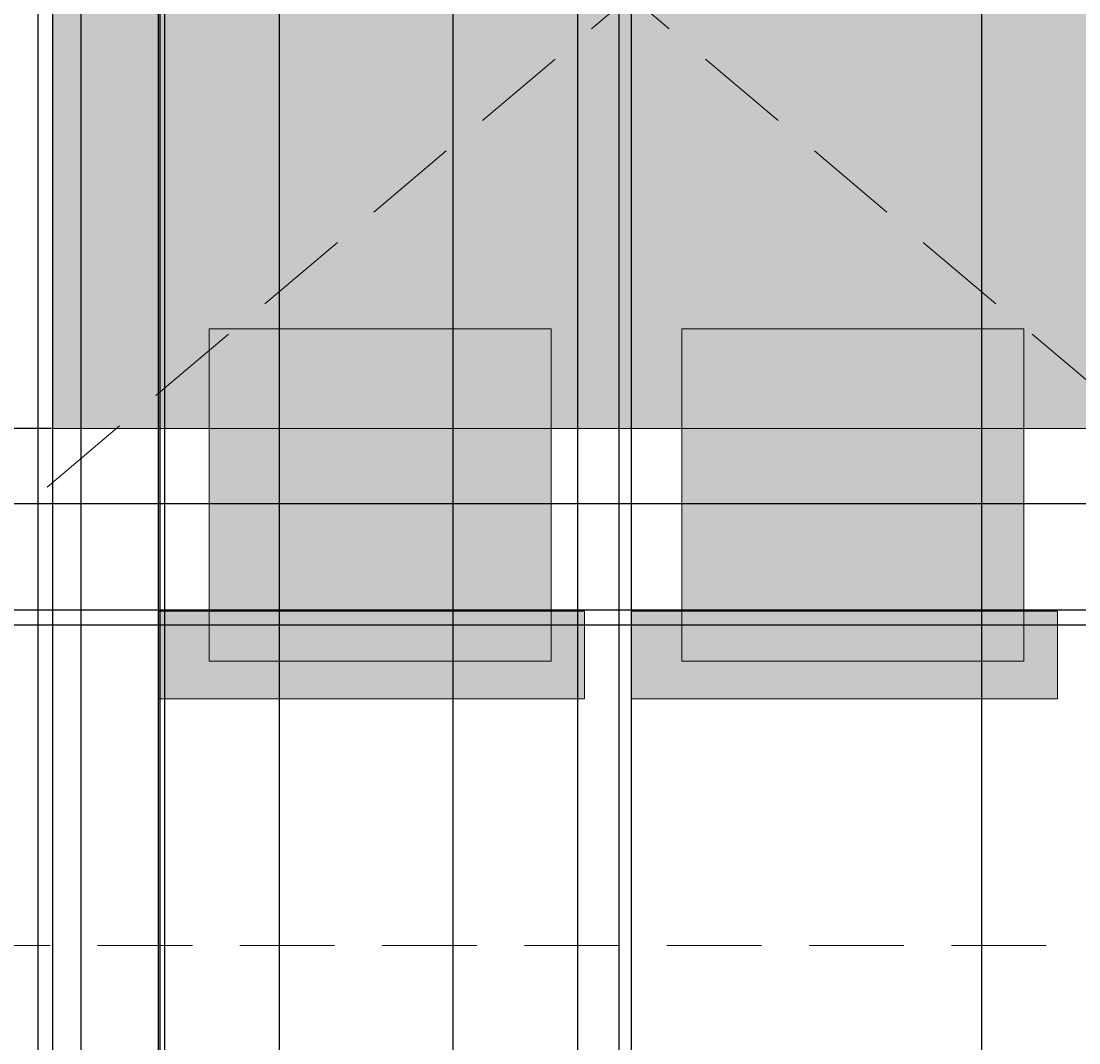
# Model space of a CAD drawing. Units: inches. Extents: x 818 to 1898, y 976 to 2364.
# Tile 69 of 96: x 1302 to 1372, y 1913 to 1980. Entities that reach past the tile are written whole.
import ezdxf

# ---------------------------------------------------------------- set-up
doc = ezdxf.new("R2010")
doc.units = ezdxf.units.IN
doc.header["$LTSCALE"] = 5
doc.header["$MEASUREMENT"] = 0
doc.linetypes.add('HIDDEN', pattern=[0.375, 0.25, -0.125])
for name, color, linetype, lineweight in [('A-ANNO-DIMS', 2, 'Continuous', 18), ('A-FLOR-OVHD', 8, 'HIDDEN', 13), ('A-FURN', 8, 'Continuous', 18), ('A-FURN-PATT', 8, 'Continuous', 9)]:
    doc.layers.add(name, color=color, linetype=linetype, lineweight=lineweight)
doc.styles.get("Standard").update_dxf_attribs({"font": 'arial.ttf'})
doc.dimstyles.get("Standard").update_dxf_attribs({"dimtxt": 0.18, "dimasz": 0.18, "dimexe": 0.18, "dimexo": 0.0625, "dimgap": 0.09, "dimtad": 0, "dimtih": 1, "dimtoh": 1, "dimdec": 4, "dimzin": 0, "dimdsep": 46, "dimtxsty": 'Standard', "dimcen": 0.09, "dimadec": 0, "dimazin": 0, "dimtfac": 1, "dimtdec": 4, "dimtofl": 0, "dimtmove": 0, "dimatfit": 3, "dimfxl": 1, "dimtolj": 1, "dimtzin": 0, "dimarcsym": 0})

# ---------------------------------------------------------------- blocks, each defined once
blk = doc.blocks.new('*D61')
at = {"layer": 'A-ANNO-DIMS', "color": 0, "lineweight": -2, "ltscale": 5, "transparency": 16777216}
for p, q in [((1071.725, 1203.027), (1071.725, 2363.873)), ((1071.905, 2363.693), (1250.936, 2363.693)), ((1430.545, 2363.693), (1251.514, 2363.693)), ((1430.725, 1203.027), (1430.725, 2363.873))]:
    blk.add_line(p, q, dxfattribs=at)
at = {"layer": 'A-ANNO-DIMS', "color": 0, "ltscale": 5, "transparency": 16777216}
for points in [[(1071.905, 2363.723), (1071.905, 2363.663), (1071.725, 2363.693)], [(1430.545, 2363.723), (1430.545, 2363.663), (1430.725, 2363.693)]]:
    blk.add_solid(points, dxfattribs=at)
at = {"layer": 'Defpoints', "color": 0, "ltscale": 5, "transparency": 16777216}
for p in [(1430.725, 2363.693), (1071.725, 1202.964), (1430.725, 1202.964)]:
    blk.add_point(p, dxfattribs=at)
at = {"layer": 'A-ANNO-DIMS', "color": 0, "ltscale": 5, "transparency": 16777216, "insert": (1251.225, 2363.693), "char_height": 0.18, "attachment_point": 5}
blk.add_mtext('\\A1;359', dxfattribs=at)
blk = doc.blocks.new('*D64')
at = {"layer": 'A-ANNO-DIMS', "color": 0, "lineweight": -2, "ltscale": 5, "transparency": 16777216}
for p, q in [((1197.725, 1501.141), (1197.725, 2363.873)), ((1197.905, 2363.693), (1313.935, 2363.693)), ((1430.545, 2363.693), (1314.516, 2363.693)), ((1430.725, 1501.141), (1430.725, 2363.873))]:
    blk.add_line(p, q, dxfattribs=at)
at = {"layer": 'A-ANNO-DIMS', "color": 0, "ltscale": 5, "transparency": 16777216}
for points in [[(1197.905, 2363.723), (1197.905, 2363.663), (1197.725, 2363.693)], [(1430.545, 2363.723), (1430.545, 2363.663), (1430.725, 2363.693)]]:
    blk.add_solid(points, dxfattribs=at)
at = {"layer": 'Defpoints', "color": 0, "ltscale": 5, "transparency": 16777216}
for p in [(1430.725, 2363.693), (1197.725, 1501.078), (1430.725, 1501.078)]:
    blk.add_point(p, dxfattribs=at)
at = {"layer": 'A-ANNO-DIMS', "color": 0, "ltscale": 5, "transparency": 16777216, "insert": (1314.225, 2363.693), "char_height": 0.18, "attachment_point": 5}
blk.add_mtext('\\A1;233', dxfattribs=at)
blk = doc.blocks.new('*D74')
at = {"layer": 'A-ANNO-DIMS', "color": 0, "lineweight": -2, "ltscale": 5, "transparency": 16777216}
for p, q in [((1590.663, 1940.078), (818.026, 1940.078)), ((818.206, 1939.898), (818.206, 1925.76)), ((818.206, 1911.258), (818.206, 1925.396)), ((1590.663, 1911.078), (818.026, 1911.078))]:
    blk.add_line(p, q, dxfattribs=at)
at = {"layer": 'A-ANNO-DIMS', "color": 0, "ltscale": 5, "transparency": 16777216}
for points in [[(818.176, 1939.898), (818.236, 1939.898), (818.206, 1940.078)], [(818.176, 1911.258), (818.236, 1911.258), (818.206, 1911.078)]]:
    blk.add_solid(points, dxfattribs=at)
at = {"layer": 'Defpoints', "color": 0, "ltscale": 5, "transparency": 16777216}
for p in [(818.206, 1940.078), (1590.725, 1940.078), (1590.725, 1911.078)]:
    blk.add_point(p, dxfattribs=at)
at = {"layer": 'A-ANNO-DIMS', "color": 0, "ltscale": 5, "transparency": 16777216, "insert": (818.206, 1925.578), "char_height": 0.18, "attachment_point": 5}
blk.add_mtext('\\A1;29', dxfattribs=at)
blk = doc.blocks.new('*D85')
at = {"layer": 'A-ANNO-DIMS', "color": 0, "lineweight": -2, "ltscale": 5, "transparency": 16777216}
for p, q in [((1258.788, 2053.078), (1897.916, 2053.078)), ((1897.736, 2052.898), (1897.736, 1876.76)), ((1897.736, 1700.258), (1897.736, 1876.396)), ((1258.788, 1700.078), (1897.916, 1700.078))]:
    blk.add_line(p, q, dxfattribs=at)
at = {"layer": 'A-ANNO-DIMS', "color": 0, "ltscale": 5, "transparency": 16777216}
for points in [[(1897.706, 2052.898), (1897.766, 2052.898), (1897.736, 2053.078)], [(1897.706, 1700.258), (1897.766, 1700.258), (1897.736, 1700.078)]]:
    blk.add_solid(points, dxfattribs=at)
at = {"layer": 'Defpoints', "color": 0, "ltscale": 5, "transparency": 16777216}
for p in [(1258.725, 2053.078), (1897.736, 2053.078), (1258.725, 1700.078)]:
    blk.add_point(p, dxfattribs=at)
at = {"layer": 'A-ANNO-DIMS', "color": 0, "ltscale": 5, "transparency": 16777216, "insert": (1897.736, 1876.578), "char_height": 0.18, "attachment_point": 5}
blk.add_mtext('\\A1;353', dxfattribs=at)
blk = doc.blocks.new('*D97')
at = {"layer": 'A-ANNO-DIMS', "color": 0, "lineweight": -2, "ltscale": 5, "transparency": 16777216}
for p, q in [((1284.17, 1071.118), (1284.17, 2363.873)), ((1284.35, 2363.693), (1310.962, 2363.693)), ((1338.361, 2363.693), (1311.749, 2363.693)), ((1338.541, 1071.118), (1338.541, 2363.873))]:
    blk.add_line(p, q, dxfattribs=at)
at = {"layer": 'A-ANNO-DIMS', "color": 0, "ltscale": 5, "transparency": 16777216}
for points in [[(1284.35, 2363.723), (1284.35, 2363.663), (1284.17, 2363.693)], [(1338.361, 2363.723), (1338.361, 2363.663), (1338.541, 2363.693)]]:
    blk.add_solid(points, dxfattribs=at)
at = {"layer": 'Defpoints', "color": 0, "ltscale": 5, "transparency": 16777216}
for p in [(1338.541, 2363.693), (1284.17, 1071.055), (1338.541, 1071.055)]:
    blk.add_point(p, dxfattribs=at)
at = {"layer": 'A-ANNO-DIMS', "color": 0, "ltscale": 5, "transparency": 16777216, "insert": (1311.355, 2363.693), "char_height": 0.18, "attachment_point": 5}
blk.add_mtext('\\A1;54.37', dxfattribs=at)
blk = doc.blocks.new('*D98')
at = {"layer": 'A-ANNO-DIMS', "color": 0, "lineweight": -2, "ltscale": 5, "transparency": 16777216}
for p, q in [((1338.541, 1071.118), (1338.541, 2363.873)), ((1338.721, 2363.693), (1364.815, 2363.693)), ((1391.696, 2363.693), (1365.602, 2363.693)), ((1391.876, 1071.118), (1391.876, 2363.873))]:
    blk.add_line(p, q, dxfattribs=at)
at = {"layer": 'A-ANNO-DIMS', "color": 0, "ltscale": 5, "transparency": 16777216}
for points in [[(1338.721, 2363.723), (1338.721, 2363.663), (1338.541, 2363.693)], [(1391.696, 2363.723), (1391.696, 2363.663), (1391.876, 2363.693)]]:
    blk.add_solid(points, dxfattribs=at)
at = {"layer": 'Defpoints', "color": 0, "ltscale": 5, "transparency": 16777216}
for p in [(1391.876, 2363.693), (1338.541, 1071.055), (1391.876, 1071.055)]:
    blk.add_point(p, dxfattribs=at)
at = {"layer": 'A-ANNO-DIMS', "color": 0, "ltscale": 5, "transparency": 16777216, "insert": (1365.208, 2363.693), "char_height": 0.18, "attachment_point": 5}
blk.add_mtext('\\A1;53.33', dxfattribs=at)
blk = doc.blocks.new('*D165')
at = {"layer": 'A-ANNO-DIMS', "color": 0, "lineweight": -2, "ltscale": 5, "transparency": 16777216}
for p, q in [((1283.818, 1510.141), (1283.818, 2363.873)), ((1283.998, 2363.693), (1324.088, 2363.693)), ((1364.966, 2363.693), (1324.876, 2363.693)), ((1365.146, 1510.141), (1365.146, 2363.873))]:
    blk.add_line(p, q, dxfattribs=at)
at = {"layer": 'A-ANNO-DIMS', "color": 0, "ltscale": 5, "transparency": 16777216}
for points in [[(1283.998, 2363.723), (1283.998, 2363.663), (1283.818, 2363.693)], [(1364.966, 2363.723), (1364.966, 2363.663), (1365.146, 2363.693)]]:
    blk.add_solid(points, dxfattribs=at)
at = {"layer": 'Defpoints', "color": 0, "ltscale": 5, "transparency": 16777216}
for p in [(1365.146, 2363.693), (1283.818, 1510.078), (1365.146, 1510.078)]:
    blk.add_point(p, dxfattribs=at)
at = {"layer": 'A-ANNO-DIMS', "color": 0, "ltscale": 5, "transparency": 16777216, "insert": (1324.482, 2363.693), "char_height": 0.18, "attachment_point": 5}
blk.add_mtext('\\A1;81.33', dxfattribs=at)
blk = doc.blocks.new('*D211')
at = {"layer": 'A-ANNO-DIMS', "color": 0, "lineweight": -2, "ltscale": 5, "transparency": 16777216}
for p, q in [((1599.66265, 1948.078237), (818.025912, 1948.078237)), ((818.205912, 1947.898237), (818.205912, 1944.758237)), ((818.205912, 1941.258237), (818.205912, 1944.398237)), ((1599.66265, 1941.078237), (818.025912, 1941.078237))]:
    blk.add_line(p, q, dxfattribs=at)
at = {"layer": 'A-ANNO-DIMS', "color": 0, "ltscale": 5, "transparency": 16777216}
for points in [[(818.175912, 1947.898237), (818.235912, 1947.898237), (818.205912, 1948.078237)], [(818.175912, 1941.258237), (818.235912, 1941.258237), (818.205912, 1941.078237)]]:
    blk.add_solid(points, dxfattribs=at)
at = {"layer": 'Defpoints', "color": 0, "ltscale": 5, "transparency": 16777216}
for p in [(818.205912, 1948.078237), (1599.72515, 1948.078237), (1599.72515, 1941.078237)]:
    blk.add_point(p, dxfattribs=at)
at = {"layer": 'A-ANNO-DIMS', "color": 0, "ltscale": 5, "transparency": 16777216, "insert": (818.205912, 1944.578237), "char_height": 0.18, "attachment_point": 5}
blk.add_mtext('\\A1;7', dxfattribs=at)
blk = doc.blocks.new('*D231')
at = {"layer": 'A-ANNO-DIMS', "color": 0, "lineweight": -2, "ltscale": 5, "transparency": 16777216}
for p, q in [((1303.931, 1952.978), (1303.931, 975.663)), ((1402.518, 1952.978), (1402.518, 975.663)), ((1304.111, 975.843), (1352.831, 975.843)), ((1402.338, 975.843), (1353.619, 975.843))]:
    blk.add_line(p, q, dxfattribs=at)
at = {"layer": 'A-ANNO-DIMS', "color": 0, "ltscale": 5, "transparency": 16777216}
for points in [[(1304.111, 975.873), (1304.111, 975.813), (1303.931, 975.843)], [(1402.338, 975.873), (1402.338, 975.813), (1402.518, 975.843)]]:
    blk.add_solid(points, dxfattribs=at)
at = {"layer": 'Defpoints', "color": 0, "ltscale": 5, "transparency": 16777216}
for p in [(1303.931, 1953.041), (1402.518, 1953.041), (1402.518, 975.843)]:
    blk.add_point(p, dxfattribs=at)
at = {"layer": 'A-ANNO-DIMS', "color": 0, "ltscale": 5, "transparency": 16777216, "insert": (1353.225, 975.843), "char_height": 0.18, "attachment_point": 5}
blk.add_mtext('\\A1;98.59', dxfattribs=at)
blk = doc.blocks.new('*D232')
at = {"layer": 'A-ANNO-DIMS', "color": 0, "lineweight": -2, "ltscale": 5, "transparency": 16777216}
for p, q in [((1303.869, 2008.392), (818.026, 2008.392)), ((818.206, 2008.212), (818.206, 1980.898)), ((818.206, 1953.221), (818.206, 1980.534)), ((1303.869, 1953.041), (818.026, 1953.041))]:
    blk.add_line(p, q, dxfattribs=at)
at = {"layer": 'A-ANNO-DIMS', "color": 0, "ltscale": 5, "transparency": 16777216}
for points in [[(818.176, 2008.212), (818.236, 2008.212), (818.206, 2008.392)], [(818.176, 1953.221), (818.236, 1953.221), (818.206, 1953.041)]]:
    blk.add_solid(points, dxfattribs=at)
at = {"layer": 'Defpoints', "color": 0, "ltscale": 5, "transparency": 16777216}
for p in [(818.206, 2008.392), (1303.931, 2008.392), (1303.931, 1953.041)]:
    blk.add_point(p, dxfattribs=at)
at = {"layer": 'A-ANNO-DIMS', "color": 0, "ltscale": 5, "transparency": 16777216, "insert": (818.206, 1980.716), "char_height": 0.18, "attachment_point": 5}
blk.add_mtext('\\A1;55.35', dxfattribs=at)
blk = doc.blocks.new('*D233')
at = {"layer": 'A-ANNO-DIMS', "color": 0, "lineweight": -2, "ltscale": 5, "transparency": 16777216}
for p, q in [((1267.725, 2044.016), (1267.725, 975.663)), ((1303.931, 2008.329), (1303.931, 975.663)), ((1267.905, 975.843), (1285.365, 975.843)), ((1303.751, 975.843), (1286.292, 975.843))]:
    blk.add_line(p, q, dxfattribs=at)
at = {"layer": 'A-ANNO-DIMS', "color": 0, "ltscale": 5, "transparency": 16777216}
for points in [[(1267.905, 975.873), (1267.905, 975.813), (1267.725, 975.843)], [(1303.751, 975.873), (1303.751, 975.813), (1303.931, 975.843)]]:
    blk.add_solid(points, dxfattribs=at)
at = {"layer": 'Defpoints', "color": 0, "ltscale": 5, "transparency": 16777216}
for p in [(1267.725, 2044.078), (1303.931, 2008.392), (1303.931, 975.843)]:
    blk.add_point(p, dxfattribs=at)
at = {"layer": 'A-ANNO-DIMS', "color": 0, "ltscale": 5, "transparency": 16777216, "insert": (1285.828, 975.843), "char_height": 0.18, "attachment_point": 5}
blk.add_mtext('\\A1;36.206', dxfattribs=at)
blk = doc.blocks.new('*D236')
at = {"layer": 'A-ANNO-DIMS', "color": 0, "lineweight": -2, "ltscale": 5, "transparency": 16777216}
for p, q in [((1310.908, 2026.145), (1310.908, 975.663)), ((1342.045, 2026.145), (1342.045, 975.663)), ((1311.088, 975.843), (1326.083, 975.843)), ((1341.865, 975.843), (1326.87, 975.843))]:
    blk.add_line(p, q, dxfattribs=at)
at = {"layer": 'A-ANNO-DIMS', "color": 0, "ltscale": 5, "transparency": 16777216}
for points in [[(1311.088, 975.873), (1311.088, 975.813), (1310.908, 975.843)], [(1341.865, 975.873), (1341.865, 975.813), (1342.045, 975.843)]]:
    blk.add_solid(points, dxfattribs=at)
at = {"layer": 'Defpoints', "color": 0, "ltscale": 5, "transparency": 16777216}
for p in [(1310.908, 2026.207), (1342.045, 2026.207), (1342.045, 975.843)]:
    blk.add_point(p, dxfattribs=at)
at = {"layer": 'A-ANNO-DIMS', "color": 0, "ltscale": 5, "transparency": 16777216, "insert": (1326.476, 975.843), "char_height": 0.18, "attachment_point": 5}
blk.add_mtext('\\A1;31.14', dxfattribs=at)
blk = doc.blocks.new('*D252')
at = {"layer": 'A-ANNO-DIMS', "color": 0, "lineweight": -2, "ltscale": 5, "transparency": 16777216}
for p, q in [((1330.305, 2053.016), (1330.305, 975.663)), ((1388.031, 2053.016), (1388.031, 975.663)), ((1330.485, 975.843), (1358.775, 975.843)), ((1387.851, 975.843), (1359.562, 975.843))]:
    blk.add_line(p, q, dxfattribs=at)
at = {"layer": 'A-ANNO-DIMS', "color": 0, "ltscale": 5, "transparency": 16777216}
for points in [[(1330.485, 975.873), (1330.485, 975.813), (1330.305, 975.843)], [(1387.851, 975.873), (1387.851, 975.813), (1388.031, 975.843)]]:
    blk.add_solid(points, dxfattribs=at)
at = {"layer": 'Defpoints', "color": 0, "ltscale": 5, "transparency": 16777216}
for p in [(1330.305, 2053.078), (1388.031, 2053.078), (1388.031, 975.843)]:
    blk.add_point(p, dxfattribs=at)
at = {"layer": 'A-ANNO-DIMS', "color": 0, "ltscale": 5, "transparency": 16777216, "insert": (1359.168, 975.843), "char_height": 0.18, "attachment_point": 5}
blk.add_mtext('\\A1;57.73', dxfattribs=at)
blk = doc.blocks.new('*D254')
at = {"layer": 'A-ANNO-DIMS', "color": 0, "lineweight": -2, "ltscale": 5, "transparency": 16777216}
for p, q in [((1267.725, 2044.016), (1267.725, 975.663)), ((1330.305, 2044.016), (1330.305, 975.663)), ((1267.905, 975.843), (1298.621, 975.843)), ((1330.125, 975.843), (1299.409, 975.843))]:
    blk.add_line(p, q, dxfattribs=at)
at = {"layer": 'A-ANNO-DIMS', "color": 0, "ltscale": 5, "transparency": 16777216}
for points in [[(1267.905, 975.873), (1267.905, 975.813), (1267.725, 975.843)], [(1330.125, 975.873), (1330.125, 975.813), (1330.305, 975.843)]]:
    blk.add_solid(points, dxfattribs=at)
at = {"layer": 'Defpoints', "color": 0, "ltscale": 5, "transparency": 16777216}
for p in [(1267.725, 2044.078), (1330.305, 2044.078), (1330.305, 975.843)]:
    blk.add_point(p, dxfattribs=at)
at = {"layer": 'A-ANNO-DIMS', "color": 0, "ltscale": 5, "transparency": 16777216, "insert": (1299.015, 975.843), "char_height": 0.18, "attachment_point": 5}
blk.add_mtext('\\A1;62.58', dxfattribs=at)
blk = doc.blocks.new('*D269')
at = {"layer": 'A-ANNO-DIMS', "color": 0, "lineweight": -2, "ltscale": 5, "transparency": 16777216}
for p, q in [((1246.938, 1534.141), (1246.938, 2363.873)), ((1247.118, 2363.693), (1293.706, 2363.693)), ((1341.079, 2363.693), (1294.491, 2363.693)), ((1341.259, 1534.141), (1341.259, 2363.873))]:
    blk.add_line(p, q, dxfattribs=at)
at = {"layer": 'A-ANNO-DIMS', "color": 0, "ltscale": 5, "transparency": 16777216}
for points in [[(1247.118, 2363.723), (1247.118, 2363.663), (1246.938, 2363.693)], [(1341.079, 2363.723), (1341.079, 2363.663), (1341.259, 2363.693)]]:
    blk.add_solid(points, dxfattribs=at)
at = {"layer": 'Defpoints', "color": 0, "ltscale": 5, "transparency": 16777216}
for p in [(1341.259, 2363.693), (1246.938, 1534.078), (1341.259, 1534.078)]:
    blk.add_point(p, dxfattribs=at)
at = {"layer": 'A-ANNO-DIMS', "color": 0, "ltscale": 5, "transparency": 16777216, "insert": (1294.099, 2363.693), "char_height": 0.18, "attachment_point": 5}
blk.add_mtext('\\A1;94.32', dxfattribs=at)
blk = doc.blocks.new('*D274')
at = {"layer": 'A-ANNO-DIMS', "color": 0, "lineweight": -2, "ltscale": 5, "transparency": 16777216}
for p, q in [((1311.025, 1897.929), (1311.025, 2363.873)), ((1311.205, 2363.693), (1344.007, 2363.693)), ((1377.599, 2363.693), (1344.797, 2363.693)), ((1377.779, 1897.929), (1377.779, 2363.873))]:
    blk.add_line(p, q, dxfattribs=at)
at = {"layer": 'A-ANNO-DIMS', "color": 0, "ltscale": 5, "transparency": 16777216}
for points in [[(1311.205, 2363.723), (1311.205, 2363.663), (1311.025, 2363.693)], [(1377.599, 2363.723), (1377.599, 2363.663), (1377.779, 2363.693)]]:
    blk.add_solid(points, dxfattribs=at)
at = {"layer": 'Defpoints', "color": 0, "ltscale": 5, "transparency": 16777216}
for p in [(1377.779, 2363.693), (1311.025, 1897.866), (1377.779, 1897.866)]:
    blk.add_point(p, dxfattribs=at)
at = {"layer": 'A-ANNO-DIMS', "color": 0, "ltscale": 5, "transparency": 16777216, "insert": (1344.402, 2363.693), "char_height": 0.18, "attachment_point": 5}
blk.add_mtext('\\A1;66.75', dxfattribs=at)
blk = doc.blocks.new('*D281')
at = {"layer": 'A-ANNO-DIMS', "color": 0, "lineweight": -2, "ltscale": 5, "transparency": 16777216}
for p, q in [((1250.303, 1913.703), (1250.303, 2363.873)), ((1250.483, 2363.693), (1420.121, 2363.693)), ((1590.545, 2363.693), (1420.907, 2363.693)), ((1590.725, 2011.141), (1590.725, 2363.873))]:
    blk.add_line(p, q, dxfattribs=at)
at = {"layer": 'A-ANNO-DIMS', "color": 0, "ltscale": 5, "transparency": 16777216}
for points in [[(1250.483, 2363.723), (1250.483, 2363.663), (1250.303, 2363.693)], [(1590.545, 2363.723), (1590.545, 2363.663), (1590.725, 2363.693)]]:
    blk.add_solid(points, dxfattribs=at)
at = {"layer": 'Defpoints', "color": 0, "ltscale": 5, "transparency": 16777216}
for p in [(1590.725, 2363.693), (1590.725, 2011.078), (1250.303, 1913.64)]:
    blk.add_point(p, dxfattribs=at)
at = {"layer": 'A-ANNO-DIMS', "color": 0, "ltscale": 5, "transparency": 16777216, "insert": (1420.514, 2363.693), "char_height": 0.18, "attachment_point": 5}
blk.add_mtext('\\A1;340.4', dxfattribs=at)
blk = doc.blocks.new('*D286')
at = {"layer": 'A-ANNO-DIMS', "color": 0, "lineweight": -2, "ltscale": 5, "transparency": 16777216}
for p, q in [((1305.828, 1851.971), (1305.828, 2363.873)), ((1306.008, 2363.693), (1308.184, 2363.693)), ((1311.147, 2363.693), (1308.971, 2363.693)), ((1311.327, 1853.812), (1311.327, 2363.873))]:
    blk.add_line(p, q, dxfattribs=at)
at = {"layer": 'A-ANNO-DIMS', "color": 0, "ltscale": 5, "transparency": 16777216}
for points in [[(1306.008, 2363.723), (1306.008, 2363.663), (1305.828, 2363.693)], [(1311.147, 2363.723), (1311.147, 2363.663), (1311.327, 2363.693)]]:
    blk.add_solid(points, dxfattribs=at)
at = {"layer": 'Defpoints', "color": 0, "ltscale": 5, "transparency": 16777216}
for p in [(1305.828, 2363.693), (1311.327, 1853.75), (1305.828, 1851.908)]:
    blk.add_point(p, dxfattribs=at)
at = {"layer": 'A-ANNO-DIMS', "color": 0, "ltscale": 5, "transparency": 16777216, "insert": (1308.577, 2363.693), "char_height": 0.18, "attachment_point": 5}
blk.add_mtext('\\A1;5.499', dxfattribs=at)
blk = doc.blocks.new('*D287')
at = {"layer": 'A-ANNO-DIMS', "color": 0, "lineweight": -2, "ltscale": 5, "transparency": 16777216}
for p, q in [((1303.869, 1953.041), (818.026, 1953.041)), ((818.206, 1952.861), (818.206, 1925.635)), ((818.206, 1898.046), (818.206, 1925.272)), ((1310.963, 1897.866), (818.026, 1897.866))]:
    blk.add_line(p, q, dxfattribs=at)
at = {"layer": 'A-ANNO-DIMS', "color": 0, "ltscale": 5, "transparency": 16777216}
for points in [[(818.176, 1952.861), (818.236, 1952.861), (818.206, 1953.041)], [(818.176, 1898.046), (818.236, 1898.046), (818.206, 1897.866)]]:
    blk.add_solid(points, dxfattribs=at)
at = {"layer": 'Defpoints', "color": 0, "ltscale": 5, "transparency": 16777216}
for p in [(818.206, 1953.041), (1303.931, 1953.041), (1311.025, 1897.866)]:
    blk.add_point(p, dxfattribs=at)
at = {"layer": 'A-ANNO-DIMS', "color": 0, "ltscale": 5, "transparency": 16777216, "insert": (818.206, 1925.454), "char_height": 0.18, "attachment_point": 5}
blk.add_mtext('\\A1;55.17', dxfattribs=at)
blk = doc.blocks.new('*D290')
at = {"layer": 'A-ANNO-DIMS', "color": 0, "lineweight": -2, "ltscale": 5, "transparency": 16777216}
for p, q in [((1302.983, 1599.435), (1302.983, 2363.873)), ((1303.163, 2363.693), (1310.57, 2363.693)), ((1318.713, 2363.693), (1311.306, 2363.693)), ((1318.893, 1607.833), (1318.893, 2363.873))]:
    blk.add_line(p, q, dxfattribs=at)
at = {"layer": 'A-ANNO-DIMS', "color": 0, "ltscale": 5, "transparency": 16777216}
for points in [[(1303.163, 2363.723), (1303.163, 2363.663), (1302.983, 2363.693)], [(1318.713, 2363.723), (1318.713, 2363.663), (1318.893, 2363.693)]]:
    blk.add_solid(points, dxfattribs=at)
at = {"layer": 'Defpoints', "color": 0, "ltscale": 5, "transparency": 16777216}
for p in [(1318.893, 2363.693), (1318.893, 1607.771), (1302.983, 1599.372)]:
    blk.add_point(p, dxfattribs=at)
at = {"layer": 'A-ANNO-DIMS', "color": 0, "ltscale": 5, "transparency": 16777216, "insert": (1310.938, 2363.693), "char_height": 0.18, "attachment_point": 5}
blk.add_mtext('\\A1;15.91', dxfattribs=at)

msp = doc.modelspace()

# ---------------------------------------------------------------- hatches: boundary and pattern name
at = {"layer": 'A-FURN-PATT', "ltscale": 5}
h = msp.add_hatch(color=256, dxfattribs=at)
h.dxf.hatch_style = 1
h.paths.add_polyline_path([(1341.9997, 1981.5338), (1317.9034, 2001.8247), (1314.2595, 2001.8247), (1314.2595, 2004.893), (1310.1046, 2008.3917), (1303.9314, 2008.3917), (1303.9314, 1953.0408), (1308.1629, 1953.0408), (1314.2595, 1958.1746), (1314.2595, 1959.6079), (1315.9616, 1959.6079)])
h.paths.add_polyline_path([(1341.9997, 1981.5338), (1315.9616, 1959.6079), (1336.7936, 1959.6079), (1336.7936, 1953.0408), (1345.3966, 1953.0408), (1345.3966, 1959.6079), (1368.0379, 1959.6079)])
h.paths.add_polyline_path([(1402.518, 2008.3917), (1398.8475, 2008.3917), (1398.8475, 2001.8247), (1376.3134, 2001.8247), (1376.3134, 2008.3917), (1373.8948, 2008.3917), (1367.9307, 2003.3695), (1367.9307, 2001.8247), (1366.0961, 2001.8247), (1341.9997, 1981.5338), (1368.0379, 1959.6079), (1375.8366, 1953.0408), (1376.3134, 1953.0408), (1376.3134, 1959.6079), (1398.8475, 1959.6079), (1398.8475, 1953.0408), (1402.518, 1953.0408)])
h.paths.add_polyline_path([(1366.0961, 2001.8247), (1345.3966, 2001.8247), (1345.3966, 2008.3917), (1336.7936, 2008.3917), (1336.7936, 2001.8247), (1317.9034, 2001.8247), (1341.9997, 1981.5338)])
h.paths.add_polyline_path([(1336.7936, 1959.6079), (1315.9616, 1959.6079), (1314.2595, 1958.1746), (1314.2595, 1953.0408), (1336.7936, 1953.0408)], flags=17)
h.paths.add_polyline_path([(1367.9307, 1959.6079), (1345.3966, 1959.6079), (1345.3966, 1953.0408), (1367.9307, 1953.0408)], flags=17)
h.paths.add_polyline_path([(1398.8475, 1959.6079), (1376.3134, 1959.6079), (1376.3134, 1953.0408), (1398.8475, 1953.0408)], flags=17)
h.paths.add_polyline_path([(1368.0379, 1959.6079), (1367.9307, 1959.6079), (1367.9307, 1953.0408), (1375.8366, 1953.0408)], flags=17)
h.paths.add_polyline_path([(1314.2595, 1958.1746), (1308.1629, 1953.0408), (1314.2595, 1953.0408)], flags=17)
h.paths.add_polyline_path([(1315.9616, 1959.6079), (1314.2595, 1959.6079), (1314.2595, 1958.1746)], flags=16)
h.paths.add_polyline_path([(1314.2595, 2008.3917), (1310.1046, 2008.3917), (1314.2595, 2004.893)], flags=17)
h.paths.add_polyline_path([(1336.7936, 2008.3917), (1314.2595, 2008.3917), (1314.2595, 2004.893), (1317.9034, 2001.8247), (1336.7936, 2001.8247)], flags=17)
h.paths.add_polyline_path([(1314.2595, 2004.893), (1314.2595, 2001.8247), (1317.9034, 2001.8247)], flags=16)
h.paths.add_polyline_path([(1367.9307, 2008.3917), (1345.3966, 2008.3917), (1345.3966, 2001.8247), (1366.0961, 2001.8247), (1367.9307, 2003.3695)], flags=17)
h.paths.add_polyline_path([(1398.8475, 2008.3917), (1376.3134, 2008.3917), (1376.3134, 2001.8247), (1398.8475, 2001.8247)], flags=17)
h.paths.add_polyline_path([(1373.8948, 2008.3917), (1367.9307, 2008.3917), (1367.9307, 2003.3695)], flags=17)
h.paths.add_polyline_path([(1367.9307, 2003.3695), (1366.0961, 2001.8247), (1367.9307, 2001.8247)], flags=16)
h.paths.add_polyline_path([(1546.1595, 2044.0782), (1451.7698, 2044.0782), (1451.7698, 2020.0782), (1546.1595, 2020.0782)])
h.paths.add_polyline_path([(1492.0729, 2040.001, 0.431429), (1491.8238, 2040.251), (1491.3087, 2040.251, 0.415217), (1491.0729, 2040.001)], flags=16)
h.paths.add_polyline_path([(1481.8346, 2039.6036), (1511.886, 2039.6036), (1511.886, 2024.9917), (1481.8346, 2024.9917)], flags=16)
h.paths.add_polyline_path([(1491.0729, 2039.4857), (1491.0729, 2039.501), (1492.0729, 2039.501, -0.4117484), (1491.8401, 2039.251), (1491.8229, 2039.251), (1491.8229, 2039.2509, 0.4325918), (1492.0729, 2039.501), (1491.0729, 2039.501, 0.432604), (1491.3229, 2039.2509), (1491.3229, 2039.251), (1491.325, 2039.251, -0.4165823)], flags=0)
h.paths.add_polyline_path([(1485.3701, 2030.9622), (1485.3701, 2034.3556, -0.4142136), (1488.3701, 2037.3556), (1490.3421, 2037.3556, -0.0779193), (1491.0729, 2038.751), (1495.0729, 2038.751, -0.3148679), (1496.07, 2037.1201, -0.3016609), (1497.9049, 2034.3556), (1497.9049, 2030.9622, -0.4142136), (1494.9049, 2027.9622), (1488.3701, 2027.9622, -0.4142136)], flags=0)
h.paths.add_polyline_path([(1490.3229, 2035.751, 0.2655648), (1491.3229, 2036.751), (1491.3229, 2037.126), (1491.0729, 2037.126, -0.7914183), (1490.5434, 2037.251, -0.7914183), (1491.0729, 2037.376), (1491.3229, 2037.376), (1491.3229, 2037.751), (1492.0729, 2037.751), (1492.0729, 2037.376), (1492.3229, 2037.376, -0.7914183), (1492.8524, 2037.251, -0.7914183), (1492.3229, 2037.126), (1492.1491, 2037.126, -0.0866263), (1492.5376, 2036.0294, 0.1070481), (1493.0729, 2035.751), (1490.3229, 2035.751)], flags=0)
h.paths.add_polyline_path([(1491.9774, 2037.251, -1), (1491.4184, 2037.251, -1)], flags=0)
h.paths.add_polyline_path([(1500.0743, 2028.6045), (1500.0743, 2029.4074), (1510.8414, 2029.4074), (1510.8414, 2028.6045)], flags=0)
h.paths.add_polyline_path([(1500.0743, 2030.5314), (1500.0743, 2031.3342), (1510.8414, 2031.3342), (1510.8414, 2030.5314)], flags=0)
h.paths.add_polyline_path([(1500.0743, 2032.94), (1500.0743, 2033.7428), (1510.8414, 2033.7428), (1510.8414, 2032.94)], flags=0)
h.paths.add_polyline_path([(1500.0743, 2035.7499), (1500.0743, 2036.5528), (1510.8414, 2036.5528), (1510.8414, 2035.7499)], flags=0)
h.paths.add_polyline_path([(1590.7251, 2044.0782), (1576.1595, 2044.0782), (1576.1595, 2020.0782), (1590.7251, 2020.0782)])
h.paths.add_polyline_path([(1668.4429, 2044.0782), (1599.7251, 2044.0782), (1599.7251, 2020.0782), (1668.4429, 2020.0782)])
h.paths.add_polyline_path([(1621.2588, 2040.001, 0.431429), (1621.0097, 2040.251), (1620.4946, 2040.251, 0.415217), (1620.2588, 2040.001)], flags=16)
h.paths.add_polyline_path([(1611.0205, 2024.9917), (1611.0205, 2039.6036), (1641.0719, 2039.6036), (1641.0719, 2024.9917)], flags=16)
h.paths.add_polyline_path([(1620.2588, 2039.4857), (1620.2588, 2039.501), (1621.2588, 2039.501, -0.4117484), (1621.026, 2039.251), (1621.0088, 2039.251), (1621.0088, 2039.2509, 0.4325918), (1621.2588, 2039.501), (1620.2588, 2039.501, 0.432604), (1620.5088, 2039.2509), (1620.5088, 2039.251), (1620.5109, 2039.251, -0.4165823)], flags=0)
h.paths.add_polyline_path([(1614.556, 2030.9622), (1614.556, 2034.3556, -0.4142136), (1617.556, 2037.3556), (1619.528, 2037.3556, -0.0779193), (1620.2588, 2038.751), (1624.2588, 2038.751, -0.3148679), (1625.2559, 2037.1201, -0.3016609), (1627.0908, 2034.3556), (1627.0908, 2030.9622, -0.4142136), (1624.0908, 2027.9622), (1617.556, 2027.9622, -0.4142136)], flags=0)
h.paths.add_polyline_path([(1619.5088, 2035.751, 0.2655648), (1620.5088, 2036.751), (1620.5088, 2037.126), (1620.2588, 2037.126, -0.7914183), (1619.7293, 2037.251, -0.7914183), (1620.2588, 2037.376), (1620.5088, 2037.376), (1620.5088, 2037.751), (1621.2588, 2037.751), (1621.2588, 2037.376), (1621.5088, 2037.376, -0.7914183), (1622.0383, 2037.251, -0.7914183), (1621.5088, 2037.126), (1621.335, 2037.126, -0.0866263), (1621.7235, 2036.0294, 0.1070481), (1622.2588, 2035.751), (1619.5088, 2035.751)], flags=0)
h.paths.add_polyline_path([(1620.6043, 2037.251, -1), (1621.1633, 2037.251, -1)], flags=0)
h.paths.add_polyline_path([(1629.2602, 2028.6045), (1629.2602, 2029.4074), (1640.0273, 2029.4074), (1640.0273, 2028.6045)], flags=0)
h.paths.add_polyline_path([(1629.2602, 2030.5314), (1629.2602, 2031.3342), (1640.0273, 2031.3342), (1640.0273, 2030.5314)], flags=0)
h.paths.add_polyline_path([(1629.2602, 2032.94), (1629.2602, 2033.7428), (1640.0273, 2033.7428), (1640.0273, 2032.94)], flags=0)
h.paths.add_polyline_path([(1629.2602, 2035.7499), (1629.2602, 2036.5528), (1640.0273, 2036.5528), (1640.0273, 2035.7499)], flags=0)
h.paths.add_polyline_path([(1705.7252, 2044.0782), (1698.4429, 2044.0782), (1698.4429, 2020.0782), (1705.7252, 2020.0782)])
h.paths.add_polyline_path([(1705.7252, 1972.0782), (1599.7251, 1972.0782), (1599.7251, 1948.0782), (1705.7252, 1948.0782)])
h.paths.add_polyline_path([(1550.0109, 1979.2444), (1483.5451, 1979.2444), (1483.5451, 1948.6602), (1550.0109, 1948.6602)])
h.paths.add_polyline_path([(1490.2586, 1948.6602), (1488.2586, 1948.6602), (1488.2586, 1941.1742, 0.4142136), (1491.2586, 1938.1742), (1500.7446, 1938.1742, -0.4142136)])
h.paths.add_polyline_path([(1513.2306, 1941.1742), (1513.2306, 1948.6602), (1511.2306, 1948.6602, -0.4142136), (1500.7446, 1938.1742), (1510.2306, 1938.1742, 0.4142136)])
h.paths.add_polyline_path([(1518.778, 1948.6602), (1516.778, 1948.6602), (1516.778, 1941.1742, 0.4142136), (1519.778, 1938.1742), (1529.264, 1938.1742, -0.4142136)])
h.paths.add_polyline_path([(1541.75, 1941.1742), (1541.75, 1948.6602), (1539.75, 1948.6602, -0.4142136), (1529.264, 1938.1742), (1538.75, 1938.1742, 0.4142136)])
h.paths.add_polyline_path([(1590.7251, 1900.0782), (1519.6413, 1900.0782), (1519.6413, 1876.0782), (1590.7251, 1876.0782)])
h = msp.add_hatch(color=256, dxfattribs=at)
h.dxf.hatch_style = 1
h.paths.add_polyline_path([(1336.7936, 1953.0408), (1314.2595, 1953.0408), (1314.2595, 1941.0096), (1336.7936, 1941.0096)])
h.paths.add_polyline_path([(1338.9915, 1941.0096), (1336.7936, 1941.0096), (1336.7936, 1937.7177), (1314.2595, 1937.7177), (1314.2595, 1941.0096), (1310.9077, 1941.0096), (1310.9077, 1935.2252), (1338.9915, 1935.2252)])
h.paths.add_polyline_path([(1336.7936, 1941.0096), (1314.2595, 1941.0096), (1314.2595, 1937.7177), (1336.7936, 1937.7177)], flags=17)
h.paths.add_polyline_path([(1367.9307, 1959.6079), (1345.3966, 1959.6079), (1345.3966, 1941.0096), (1367.9307, 1941.0096)])
h.paths.add_polyline_path([(1398.8475, 1953.0408), (1376.3134, 1953.0408), (1376.3134, 1952.6393), (1390.1242, 1941.0096), (1398.8475, 1941.0096)])
h.paths.add_polyline_path([(1376.3134, 1952.6393), (1376.3134, 1941.0096), (1390.1242, 1941.0096)], flags=17)
h.paths.add_polyline_path([(1370.1286, 1941.0096), (1367.9307, 1941.0096), (1367.9307, 1937.7177), (1345.3966, 1937.7177), (1345.3966, 1941.0096), (1342.0448, 1941.0096), (1342.0448, 1935.2252), (1370.1286, 1935.2252)])
h.paths.add_polyline_path([(1367.9307, 1941.0096), (1345.3966, 1941.0096), (1345.3966, 1937.7177), (1367.9307, 1937.7177)], flags=17)
h.paths.add_polyline_path([(1390.1242, 1941.0096), (1376.3134, 1941.0096), (1376.3134, 1937.7177), (1394.0336, 1937.7177)], flags=17)
h.paths.add_polyline_path([(1394.0336, 1937.7177), (1376.3134, 1937.7177), (1376.3134, 1941.0096), (1372.9616, 1941.0096), (1372.9616, 1935.2252), (1396.9935, 1935.2252)])
h.paths.add_polyline_path([(1398.8475, 1941.0096), (1390.1242, 1941.0096), (1394.0336, 1937.7177), (1398.8475, 1937.7177)])
h.paths.add_polyline_path([(1401.0455, 1941.0096), (1398.8475, 1941.0096), (1398.8475, 1937.7177), (1394.0336, 1937.7177), (1396.9935, 1935.2252), (1401.0455, 1935.2252)])
h.paths.add_polyline_path([(1336.7936, 2020.4229), (1314.2595, 2020.4229), (1314.2595, 2008.3917), (1336.7936, 2008.3917)])
h.paths.add_polyline_path([(1336.7936, 2023.7149), (1314.2595, 2023.7149), (1314.2595, 2020.4229), (1336.7936, 2020.4229)], flags=17)
h.paths.add_polyline_path([(1338.9915, 2026.2074), (1310.9077, 2026.2074), (1310.9077, 2020.4229), (1314.2595, 2020.4229), (1314.2595, 2023.7149), (1336.7936, 2023.7149), (1336.7936, 2020.4229), (1338.9915, 2020.4229)])
h.paths.add_polyline_path([(1367.9307, 2023.7149), (1345.3966, 2023.7149), (1345.3966, 2020.4229), (1367.9307, 2020.4229)], flags=17)
h.paths.add_polyline_path([(1370.1286, 2026.2074), (1342.0448, 2026.2074), (1342.0448, 2020.4229), (1345.3966, 2020.4229), (1345.3966, 2023.7149), (1367.9307, 2023.7149), (1367.9307, 2020.4229), (1370.1286, 2020.4229)])
h.paths.add_polyline_path([(1367.9307, 2020.4229), (1345.3966, 2020.4229), (1345.3966, 2008.3917), (1367.9307, 2008.3917)])
h.paths.add_polyline_path([(1398.8475, 2020.4229), (1388.1824, 2020.4229), (1376.3134, 2010.4284), (1376.3134, 2008.3917), (1398.8475, 2008.3917)])
h.paths.add_polyline_path([(1392.0918, 2023.7149), (1376.3134, 2023.7149), (1376.3134, 2020.4229), (1388.1824, 2020.4229)], flags=17)
h.paths.add_polyline_path([(1388.1824, 2020.4229), (1376.3134, 2020.4229), (1376.3134, 2010.4284)], flags=17)
h.paths.add_polyline_path([(1395.0518, 2026.2074), (1372.9616, 2026.2074), (1372.9616, 2020.4229), (1376.3134, 2020.4229), (1376.3134, 2023.7149), (1392.0918, 2023.7149)])
h.paths.add_polyline_path([(1398.8475, 2023.7149), (1392.0918, 2023.7149), (1388.1824, 2020.4229), (1398.8475, 2020.4229)])
h.paths.add_polyline_path([(1401.0455, 2026.2074), (1395.0518, 2026.2074), (1392.0918, 2023.7149), (1398.8475, 2023.7149), (1398.8475, 2020.4229), (1401.0455, 2020.4229)])
h.paths.add_polyline_path([(1327.0339, 1897.8663), (1311.025, 1897.8663), (1311.025, 1876.0782), (1327.0339, 1876.0782)])
h.paths.add_polyline_path([(1377.7791, 1897.8663), (1359.9579, 1897.8663), (1359.9579, 1876.0782), (1377.7791, 1876.0782)])
h.paths.add_polyline_path([(1430.7251, 1541.0439), (1406.7252, 1541.0439), (1406.7252, 1525.9965), (1430.7251, 1525.9965)])
h.paths.add_polyline_path([(1430.7251, 1587.4164), (1406.7252, 1587.4164), (1406.7252, 1570.9187), (1430.7251, 1570.9187)])

# ---------------------------------------------------------------- linework, layer by layer
at = {"layer": 'A-FLOR-OVHD', "ltscale": 5}
for p, q in [((1416.2743, 1918.9894), (1267.7251, 2044.0782)), ((1267.7251, 1918.9894), (1416.2743, 2044.0782))]:
    msp.add_line(p, q, dxfattribs=at)
msp.add_lwpolyline([(1267.7251, 2044.0782), (1416.2743, 2044.0782), (1416.2743, 1918.9894), (1267.7251, 1918.9894)], close=True, dxfattribs=at)
at = {"layer": 'A-FURN'}
for points in [[(1303.9314, 2008.3917), (1402.518, 2008.3917), (1402.518, 1953.0408), (1303.9314, 1953.0408)], [(1314.2595, 1959.6079), (1336.7936, 1959.6079), (1336.7936, 1937.7177), (1314.2595, 1937.7177)], [(1345.3966, 1959.6079), (1367.9307, 1959.6079), (1367.9307, 1937.7177), (1345.3966, 1937.7177)], [(1310.9077, 1941.0096), (1338.9915, 1941.0096), (1338.9915, 1935.2252), (1310.9077, 1935.2252)], [(1342.0448, 1941.0096), (1370.1286, 1941.0096), (1370.1286, 1935.2252), (1342.0448, 1935.2252)]]:
    msp.add_lwpolyline(points, close=True, dxfattribs=at)

# ---------------------------------------------------------------- dimensions: what is measured, and where the dimension line sits
at = {"layer": 'A-ANNO-DIMS', "ltscale": 5}
for base, p1, p2, override, picture, middle in [((1430.7251, 2363.6929), (1071.7251, 1202.9642), (1430.7251, 1202.9642), {"dimdec": 0, "dimlfac": 1, "dimrnd": 0, "dimzin": 0, "dimdsep": 46, "dimlunit": 2}, '*D61', (1251.2251, 2363.6929)), ((1430.7251, 2363.6929), (1197.7251, 1501.0782), (1430.7251, 1501.0782), {"dimdec": 0, "dimlfac": 1, "dimrnd": 0, "dimzin": 0, "dimdsep": 46, "dimlunit": 2}, '*D64', (1314.2251, 2363.6929)), ((1341.2593, 2363.6929), (1246.9377, 1534.0782), (1341.2593, 1534.0782), {"dimdec": 2, "dimlfac": 1, "dimrnd": 0, "dimzin": 0, "dimdsep": 46, "dimlunit": 2}, '*D269', (1294.0985, 2363.6929)), ((1590.7251, 2363.6929), (1250.3029, 1913.6401), (1590.7251, 2011.0782), {"dimdec": 1, "dimlfac": 1, "dimrnd": 0, "dimzin": 0, "dimdsep": 46, "dimlunit": 2}, '*D281', (1420.514, 2363.6929)), ((1365.1463, 2363.6929), (1283.8183, 1510.0782), (1365.1463, 1510.0782), {"dimdec": 2, "dimlfac": 1, "dimrnd": 0, "dimzin": 0, "dimdsep": 46, "dimlunit": 2}, '*D165', (1324.4823, 2363.6929)), ((1338.5412, 2363.6929), (1284.1697, 1071.0552), (1338.5412, 1071.0552), {"dimdec": 2, "dimlfac": 1, "dimrnd": 0, "dimzin": 0, "dimdsep": 46, "dimlunit": 2}, '*D97', (1311.3554, 2363.6929)), ((1318.8931, 2363.6929), (1302.9835, 1599.3725), (1318.8931, 1607.7707), {"dimdec": 2, "dimlfac": 1, "dimrnd": 0, "dimzin": 0, "dimdsep": 46, "dimlunit": 2}, '*D290', (1310.9383, 2363.6929)), ((1305.8278, 2363.6929), (1311.3271, 1853.7496), (1305.8278, 1851.9081), {"dimdec": 3, "dimlfac": 1, "dimrnd": 0, "dimzin": 0, "dimdsep": 46, "dimlunit": 2}, '*D286', (1308.5774, 2363.6929)), ((1377.7791, 2363.6929), (1311.025, 1897.8663), (1377.7791, 1897.8663), {"dimdec": 2, "dimlfac": 1, "dimrnd": 0, "dimzin": 0, "dimdsep": 46, "dimlunit": 2}, '*D274', (1344.4021, 2363.6929)), ((1391.8757, 2363.6929), (1338.5412, 1071.0552), (1391.8757, 1071.0552), {"dimdec": 2, "dimlfac": 1, "dimrnd": 0, "dimzin": 0, "dimdsep": 46, "dimlunit": 2}, '*D98', (1365.2084, 2363.6929)), ((1388.0315, 975.8433), (1330.305, 2053.0782), (1388.0315, 2053.0782), {"dimdec": 2, "dimlfac": 1, "dimrnd": 0, "dimzin": 0, "dimdsep": 46, "dimlunit": 2}, '*D252', (1359.1682, 975.8433)), ((1303.9314, 975.8433), (1267.7251, 2044.0782), (1303.9314, 2008.3917), {"dimdec": 3, "dimlfac": 1, "dimrnd": 0, "dimzin": 0, "dimdsep": 46, "dimlunit": 2}, '*D233', (1285.8283, 975.8433)), ((1330.305, 975.8433), (1267.7251, 2044.0782), (1330.305, 2044.0782), {"dimdec": 2, "dimlfac": 1, "dimrnd": 0, "dimzin": 0, "dimdsep": 46, "dimlunit": 2}, '*D254', (1299.0151, 975.8433)), ((1342.0448, 975.8433), (1310.9077, 2026.2074), (1342.0448, 2026.2074), {"dimdec": 2, "dimlfac": 1, "dimrnd": 0, "dimzin": 0, "dimdsep": 46, "dimlunit": 2}, '*D236', (1326.4762, 975.8433)), ((1402.518, 975.8433), (1303.9314, 1953.0408), (1402.518, 1953.0408), {"dimdec": 2, "dimlfac": 1, "dimrnd": 0, "dimzin": 0, "dimdsep": 46, "dimlunit": 2}, '*D231', (1353.2247, 975.8433))]:
    dim = msp.add_linear_dim(base=base, p1=p1, p2=p2, dimstyle='Standard', override=override, dxfattribs=at)
    dim.commit()
    dim.dimension.update_dxf_attribs({"geometry": picture, "text_midpoint": middle})
for base, p1, p2, override, picture, middle in [((1897.736, 2053.0782), (1258.7251, 1700.0782), (1258.7251, 2053.0782), {"dimdec": 0, "dimlfac": 1, "dimrnd": 0, "dimzin": 0, "dimdsep": 46, "dimlunit": 2}, '*D85', (1897.736, 1876.5782)), ((818.2059, 2008.3917), (1303.9314, 1953.0408), (1303.9314, 2008.3917), {"dimdec": 2, "dimlfac": 1, "dimrnd": 0, "dimzin": 0, "dimdsep": 46, "dimlunit": 2}, '*D232', (818.2059, 1980.7163)), ((818.2059, 1953.0408), (1311.025, 1897.8663), (1303.9314, 1953.0408), {"dimdec": 2, "dimlfac": 1, "dimrnd": 0, "dimzin": 0, "dimdsep": 46, "dimlunit": 2}, '*D287', (818.2059, 1925.4536)), ((818.2059, 1948.0782), (1599.7251, 1941.0782), (1599.7251, 1948.0782), {"dimdec": 0, "dimlfac": 1, "dimrnd": 0, "dimzin": 0, "dimdsep": 46, "dimlunit": 2}, '*D211', (818.2059, 1944.5782)), ((818.2059, 1940.0782), (1590.7251, 1911.0782), (1590.7251, 1940.0782), {"dimdec": 0, "dimlfac": 1, "dimrnd": 0, "dimzin": 0, "dimdsep": 46, "dimlunit": 2}, '*D74', (818.2059, 1925.5782))]:
    dim = msp.add_linear_dim(base=base, p1=p1, p2=p2, angle=90, dimstyle='Standard', override=override, dxfattribs=at)
    dim.commit()
    dim.dimension.update_dxf_attribs({"geometry": picture, "text_midpoint": middle})

doc.saveas('drawing.dxf')
